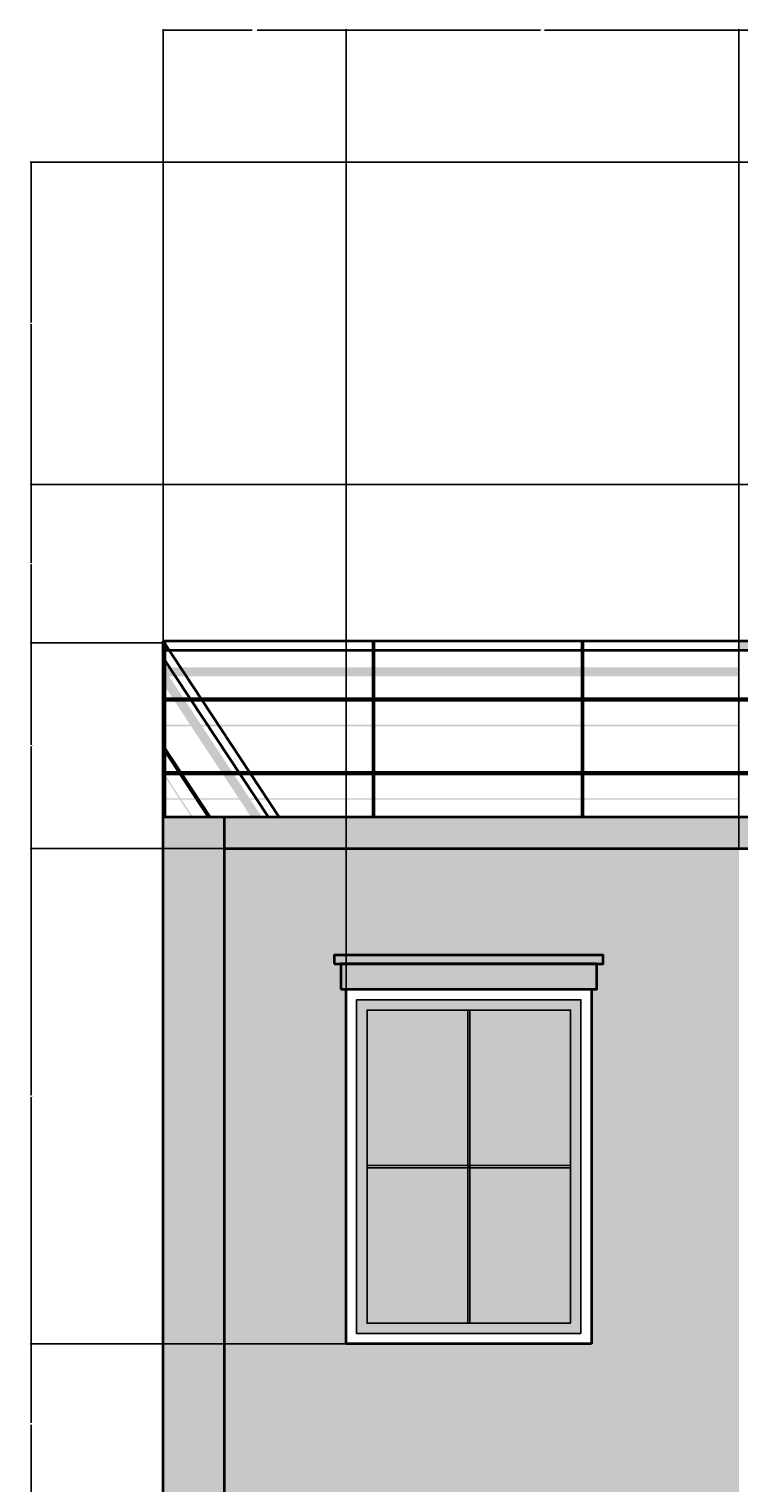
# Model space of a CAD drawing. Units: feet. Extents: x 2415 to 6174, y 866 to 1295.
# Tile 2 of 9: x 3227 to 3364, y 1016 to 1295. Entities that reach past the tile are written whole.
import ezdxf

# ---------------------------------------------------------------- set-up
doc = ezdxf.new("R2010")
doc.units = ezdxf.units.FT
for name, color, linetype, lineweight in [('A-ANNO-DIMS', 2, 'Continuous', 18), ('A-ELEV', 7, 'Continuous', 35), ('A-ELEV-PATT', 8, 'Continuous', 13), ('A-GLAZ', 4, 'Continuous', 25)]:
    doc.layers.add(name, color=color, linetype=linetype, lineweight=lineweight)
doc.styles.get("Standard").update_dxf_attribs({"font": 'arial.ttf'})
doc.dimstyles.get("Standard").update_dxf_attribs({"dimtxt": 0.18, "dimasz": 0.18, "dimexe": 0.18, "dimexo": 0.0625, "dimgap": 0.09, "dimtad": 0, "dimtih": 1, "dimtoh": 1, "dimdec": 1, "dimzin": 0, "dimdsep": 46, "dimlunit": 3, "dimtxsty": 'Standard', "dimcen": 0.09, "dimadec": 0, "dimazin": 0, "dimtfac": 1, "dimtdec": 1, "dimtofl": 0, "dimtmove": 0, "dimatfit": 3, "dimfxl": 1, "dimtolj": 1, "dimtzin": 0, "dimarcsym": 0})

# ---------------------------------------------------------------- blocks, each defined once
blk = doc.blocks.new('WIN-SMALL')
for points in [[(3333.49, 1044.32), (3290.35, 1044.32), (3290.35, 1108.53), (3333.49, 1108.53)], [(3331.49, 1046.32), (3292.35, 1046.32), (3292.35, 1106.53), (3331.49, 1106.53)], [(3311.72, 1106.53), (3312.12, 1106.53), (3312.12, 1046.32), (3311.72, 1046.32)]]:
    blk.add_lwpolyline(points, close=True)
for points in [[(3292.35, 1076.62), (3331.49, 1076.62)], [(3331.49, 1076.22), (3292.35, 1076.22)]]:
    blk.add_lwpolyline(points)
blk = doc.blocks.new('*D61')
at = {"layer": 'A-ANNO-DIMS', "color": 0, "lineweight": -2, "transparency": 16777216}
for p, q in [((3253.13, 1177.2), (3253.13, 1295.18)), ((3253.31, 1295), (3270.27, 1295)), ((3288.17, 1295), (3271.2, 1295)), ((3288.35, 1042.38), (3288.35, 1295.18))]:
    blk.add_line(p, q, dxfattribs=at)
at = {"layer": 'A-ANNO-DIMS', "color": 0, "transparency": 16777216}
for points in [[(3253.31, 1295.03), (3253.31, 1294.97), (3253.13, 1295)], [(3288.17, 1295.03), (3288.17, 1294.97), (3288.35, 1295)]]:
    blk.add_solid(points, dxfattribs=at)
at = {"layer": 'Defpoints', "color": 0, "transparency": 16777216}
for p in [(3288.35, 1295), (3253.13, 1177.14), (3288.35, 1042.32)]:
    blk.add_point(p, dxfattribs=at)
at = {"layer": 'A-ANNO-DIMS', "color": 0, "transparency": 16777216, "insert": (3270.74, 1295), "char_height": 0.18, "attachment_point": 5}
blk.add_mtext('\\A1;35.216', dxfattribs=at)
blk = doc.blocks.new('*D62')
at = {"layer": 'A-ANNO-DIMS', "color": 0, "lineweight": -2, "transparency": 16777216}
for p, q in [((3288.35, 1042.38), (3288.35, 1295.18)), ((3288.53, 1295), (3325.71, 1295)), ((3363.69, 1295), (3326.5, 1295)), ((3363.87, 1137.66), (3363.87, 1295.18))]:
    blk.add_line(p, q, dxfattribs=at)
at = {"layer": 'A-ANNO-DIMS', "color": 0, "transparency": 16777216}
for points in [[(3288.53, 1295.03), (3288.53, 1294.97), (3288.35, 1295)], [(3363.69, 1295.03), (3363.69, 1294.97), (3363.87, 1295)]]:
    blk.add_solid(points, dxfattribs=at)
at = {"layer": 'Defpoints', "color": 0, "transparency": 16777216}
for p in [(3363.87, 1295), (3363.87, 1137.6), (3288.35, 1042.32)]:
    blk.add_point(p, dxfattribs=at)
at = {"layer": 'A-ANNO-DIMS', "color": 0, "transparency": 16777216, "insert": (3326.11, 1295), "char_height": 0.18, "attachment_point": 5}
blk.add_mtext('\\A1;75.52', dxfattribs=at)
blk = doc.blocks.new('*D63')
at = {"layer": 'A-ANNO-DIMS', "color": 0, "lineweight": -2, "transparency": 16777216}
for p, q in [((3363.87, 1137.66), (3363.87, 1295.18)), ((3364.05, 1295), (3414.78, 1295)), ((3466.42, 1295), (3415.69, 1295)), ((3466.6, 1137.66), (3466.6, 1295.18))]:
    blk.add_line(p, q, dxfattribs=at)
at = {"layer": 'A-ANNO-DIMS', "color": 0, "transparency": 16777216}
for points in [[(3364.05, 1295.03), (3364.05, 1294.97), (3363.87, 1295)], [(3466.42, 1295.03), (3466.42, 1294.97), (3466.6, 1295)]]:
    blk.add_solid(points, dxfattribs=at)
at = {"layer": 'Defpoints', "color": 0, "transparency": 16777216}
for p in [(3466.6, 1295), (3363.87, 1137.6), (3466.6, 1137.6)]:
    blk.add_point(p, dxfattribs=at)
at = {"layer": 'A-ANNO-DIMS', "color": 0, "transparency": 16777216, "insert": (3415.23, 1295), "char_height": 0.18, "attachment_point": 5}
blk.add_mtext('\\A1;102.73', dxfattribs=at)
blk = doc.blocks.new('*D74')
at = {"layer": 'A-ANNO-DIMS', "color": 0, "lineweight": -2, "transparency": 16777216}
for p, q in [((3288.28, 1042.32), (3227.55, 1042.32)), ((3227.73, 1042.14), (3227.73, 1027.14)), ((3227.73, 1011.78), (3227.73, 1026.78)), ((3264.85, 1011.6), (3227.55, 1011.6))]:
    blk.add_line(p, q, dxfattribs=at)
at = {"layer": 'A-ANNO-DIMS', "color": 0, "transparency": 16777216}
for points in [[(3227.7, 1042.14), (3227.76, 1042.14), (3227.73, 1042.32)], [(3227.7, 1011.78), (3227.76, 1011.78), (3227.73, 1011.6)]]:
    blk.add_solid(points, dxfattribs=at)
at = {"layer": 'Defpoints', "color": 0, "transparency": 16777216}
for p in [(3227.73, 1042.32), (3288.35, 1042.32), (3264.92, 1011.6)]:
    blk.add_point(p, dxfattribs=at)
at = {"layer": 'A-ANNO-DIMS', "color": 0, "transparency": 16777216, "insert": (3227.73, 1026.96), "char_height": 0.18, "attachment_point": 5}
blk.add_mtext('\\A1;30.72', dxfattribs=at)
blk = doc.blocks.new('*D75')
at = {"layer": 'A-ANNO-DIMS', "color": 0, "lineweight": -2, "transparency": 16777216}
for p, q in [((3363.8, 1137.6), (3227.55, 1137.6)), ((3227.73, 1137.42), (3227.73, 1090.14)), ((3227.73, 1042.5), (3227.73, 1089.78)), ((3288.28, 1042.32), (3227.55, 1042.32))]:
    blk.add_line(p, q, dxfattribs=at)
at = {"layer": 'A-ANNO-DIMS', "color": 0, "transparency": 16777216}
for points in [[(3227.7, 1137.42), (3227.76, 1137.42), (3227.73, 1137.6)], [(3227.7, 1042.5), (3227.76, 1042.5), (3227.73, 1042.32)]]:
    blk.add_solid(points, dxfattribs=at)
at = {"layer": 'Defpoints', "color": 0, "transparency": 16777216}
for p in [(3227.73, 1137.6), (3363.87, 1137.6), (3288.35, 1042.32)]:
    blk.add_point(p, dxfattribs=at)
at = {"layer": 'A-ANNO-DIMS', "color": 0, "transparency": 16777216, "insert": (3227.73, 1089.96), "char_height": 0.18, "attachment_point": 5}
blk.add_mtext('\\A1;95.28', dxfattribs=at)
blk = doc.blocks.new('*D76')
at = {"layer": 'A-ANNO-DIMS', "color": 0, "lineweight": -2, "transparency": 16777216}
for p, q in [((3253.07, 1177.14), (3227.55, 1177.14)), ((3227.73, 1176.96), (3227.73, 1157.55)), ((3227.73, 1137.78), (3227.73, 1157.19)), ((3363.8, 1137.6), (3227.55, 1137.6))]:
    blk.add_line(p, q, dxfattribs=at)
at = {"layer": 'A-ANNO-DIMS', "color": 0, "transparency": 16777216}
for points in [[(3227.7, 1176.96), (3227.76, 1176.96), (3227.73, 1177.14)], [(3227.7, 1137.78), (3227.76, 1137.78), (3227.73, 1137.6)]]:
    blk.add_solid(points, dxfattribs=at)
at = {"layer": 'Defpoints', "color": 0, "transparency": 16777216}
for p in [(3227.73, 1177.14), (3253.13, 1177.14), (3363.87, 1137.6)]:
    blk.add_point(p, dxfattribs=at)
at = {"layer": 'A-ANNO-DIMS', "color": 0, "transparency": 16777216, "insert": (3227.73, 1157.37), "char_height": 0.18, "attachment_point": 5}
blk.add_mtext('\\A1;39.54', dxfattribs=at)
blk = doc.blocks.new('*D77')
at = {"layer": 'A-ANNO-DIMS', "color": 0, "lineweight": -2, "transparency": 16777216}
for p, q in [((3506.73, 1207.6), (3227.55, 1207.6)), ((3227.73, 1207.42), (3227.73, 1192.55)), ((3227.73, 1177.32), (3227.73, 1192.19)), ((3253.07, 1177.14), (3227.55, 1177.14))]:
    blk.add_line(p, q, dxfattribs=at)
at = {"layer": 'A-ANNO-DIMS', "color": 0, "transparency": 16777216}
for points in [[(3227.7, 1207.42), (3227.76, 1207.42), (3227.73, 1207.6)], [(3227.7, 1177.32), (3227.76, 1177.32), (3227.73, 1177.14)]]:
    blk.add_solid(points, dxfattribs=at)
at = {"layer": 'Defpoints', "color": 0, "transparency": 16777216}
for p in [(3227.73, 1207.6), (3506.79, 1207.6), (3253.13, 1177.14)]:
    blk.add_point(p, dxfattribs=at)
at = {"layer": 'A-ANNO-DIMS', "color": 0, "transparency": 16777216, "insert": (3227.73, 1192.37), "char_height": 0.18, "attachment_point": 5}
blk.add_mtext('\\A1;30.457', dxfattribs=at)
blk = doc.blocks.new('*D78')
at = {"layer": 'A-ANNO-DIMS', "color": 0, "lineweight": -2, "transparency": 16777216}
for p, q in [((3571.87, 1269.6), (3227.55, 1269.6)), ((3227.73, 1269.42), (3227.73, 1238.78)), ((3227.73, 1207.78), (3227.73, 1238.42)), ((3506.73, 1207.6), (3227.55, 1207.6))]:
    blk.add_line(p, q, dxfattribs=at)
at = {"layer": 'A-ANNO-DIMS', "color": 0, "transparency": 16777216}
for points in [[(3227.7, 1269.42), (3227.76, 1269.42), (3227.73, 1269.6)], [(3227.7, 1207.78), (3227.76, 1207.78), (3227.73, 1207.6)]]:
    blk.add_solid(points, dxfattribs=at)
at = {"layer": 'Defpoints', "color": 0, "transparency": 16777216}
for p in [(3227.73, 1269.6), (3571.93, 1269.6), (3506.79, 1207.6)]:
    blk.add_point(p, dxfattribs=at)
at = {"layer": 'A-ANNO-DIMS', "color": 0, "transparency": 16777216, "insert": (3227.73, 1238.6), "char_height": 0.18, "attachment_point": 5}
blk.add_mtext('\\A1;62', dxfattribs=at)

msp = doc.modelspace()

# ---------------------------------------------------------------- hatches: boundary and pattern name
at = {"layer": 'A-ELEV-PATT'}
h = msp.add_hatch(color=256, dxfattribs=at)
h.set_gradient(color1=(255, 255, 255), tint=1)
h.paths.add_polyline_path([(3264.916, 1143.5993), (3253.129, 1143.5993), (3253.129, 891.5993), (3264.916, 891.5993)])
h.paths.add_polyline_path([(3470.0448, 1143.5993), (3264.916, 1143.5993), (3264.916, 1137.5992), (3466.5999, 1137.5992)])
h.paths.add_polyline_path([(3363.8667, 1137.5992), (3264.916, 1137.5992), (3264.916, 1011.5992), (3363.8667, 1011.5992)])
h.paths.add_polyline_path([(3286.0429, 1117.0591), (3337.7904, 1117.0591), (3337.7904, 1115.4381), (3336.5314, 1115.4381), (3336.5314, 1110.528), (3335.4882, 1110.528), (3335.4882, 1042.3194), (3288.3452, 1042.3194), (3288.3452, 1110.528), (3287.3019, 1110.528), (3287.3019, 1115.4381), (3286.0429, 1115.4381)], flags=16)
h.paths.add_polyline_path([(3290.3452, 1108.528), (3333.4882, 1108.528), (3333.4882, 1044.3194), (3290.3452, 1044.3194)], flags=0)
h.paths.add_polyline_path([(3292.3452, 1106.528), (3331.4882, 1106.528), (3331.4882, 1046.3194), (3292.3452, 1046.3194)], flags=0)
h.paths.add_polyline_path([(3311.7156, 1106.528), (3312.1178, 1106.528), (3312.1178, 1046.3194), (3311.7156, 1046.3194)], flags=0)
h.paths.add_polyline_path([(3682.0722, 1263.5993), (3578.5579, 1263.5993), (3578.5579, 1137.5992), (3578.5579, 961.3655), (3682.0722, 961.3655)])
h.paths.add_polyline_path([(3660.8129, 1239.0671), (3660.8129, 996.6447), (3602.2151, 996.6447), (3602.2151, 1239.0671)], flags=16)
h.paths.add_polyline_path([(3632.2447, 1239.0671), (3632.2447, 996.6447), (3630.7833, 996.6447), (3630.7833, 1029.3019), (3602.2151, 1029.3019), (3602.2151, 1030.7632), (3630.7833, 1030.7632), (3630.7833, 1071.2549), (3602.2151, 1071.2549), (3602.2151, 1072.7163), (3630.7833, 1072.7163), (3630.7833, 1113.2079), (3602.2151, 1113.2079), (3602.2151, 1114.6693), (3630.7833, 1114.6693), (3630.7833, 1155.161), (3602.2151, 1155.161), (3602.2151, 1156.6224), (3630.7833, 1156.6224), (3630.7833, 1197.114), (3602.2151, 1197.114), (3602.2151, 1198.5754), (3630.7833, 1198.5754), (3630.7833, 1239.0671)], flags=0)
h.paths.add_polyline_path([(3733.129, 951.5993), (3634.5374, 951.5993), (3634.5374, 891.5993), (3733.129, 891.5993)])
h.paths.add_polyline_path([(3627.8799, 951.5993), (3621.0953, 951.5993), (3621.0953, 891.5993), (3627.8799, 891.5993)])
h.paths.add_polyline_path([(3614.4378, 951.5993), (3607.6532, 951.5993), (3607.6532, 891.5993), (3614.4378, 891.5993)])
h.paths.add_polyline_path([(3565.9347, 951.5993), (3441.3079, 951.5993), (3441.3079, 891.5993), (3565.9347, 891.5993)], flags=17)
h.paths.add_polyline_path([(3571.9347, 957.5993), (3435.3079, 957.5993), (3435.3079, 891.5993), (3441.3079, 891.5993), (3441.3079, 951.5993), (3565.9347, 951.5993), (3565.9347, 891.5993), (3571.9347, 891.5993)])
h.paths.add_polyline_path([(3435.3079, 1011.5992), (3423.5209, 1011.5992), (3423.5209, 891.5993), (3435.3079, 891.5993), (3435.3079, 957.5993)])
h.paths.add_polyline_path([(3690.0912, 1269.5992), (3571.9347, 1269.5992), (3571.9347, 1263.5993), (3690.0912, 1263.5993)])
h.paths.add_polyline_path([(3571.9347, 1269.5992), (3538.5122, 1257.6449), (3538.5122, 1251.6449), (3571.9347, 1263.5993)])
h = msp.add_hatch(color=256, dxfattribs=at)
h.set_gradient(color2=(0, 0, 0))
h.paths.add_polyline_path([(3489.4854, 1177.4585), (3454.5146, 1177.4585), (3454.5146, 1175.7117), (3488.4825, 1175.7117)])
h.paths.add_polyline_path([(3454.5146, 1177.4585), (3454.2507, 1177.4585), (3454.2507, 1175.7117), (3454.5146, 1175.7117)])
h.paths.add_polyline_path([(3454.5146, 1175.7117), (3454.2507, 1175.7117), (3454.2507, 1166.3873), (3454.5146, 1166.3873)])
h.paths.add_polyline_path([(3454.5146, 1166.3873), (3454.2507, 1166.3873), (3454.2507, 1166.1234), (3454.5146, 1166.1234)])
h.paths.add_polyline_path([(3483.1288, 1166.3873), (3454.5146, 1166.3873), (3454.5146, 1166.1234), (3482.9773, 1166.1234)])
h.paths.add_polyline_path([(3454.2507, 1166.3873), (3414.3148, 1166.3873), (3414.3148, 1166.1234), (3454.2507, 1166.1234)])
h.paths.add_polyline_path([(3454.5146, 1166.1234), (3454.2507, 1166.1234), (3454.2507, 1152.2269), (3454.5146, 1152.2269)])
h.paths.add_polyline_path([(3454.5146, 1152.2269), (3454.2507, 1152.2269), (3454.2507, 1151.963), (3454.5146, 1151.963)])
h.paths.add_polyline_path([(3474.9985, 1152.2269), (3454.5146, 1152.2269), (3454.5146, 1151.963), (3474.8469, 1151.963)])
h.paths.add_polyline_path([(3454.2507, 1152.2269), (3414.3148, 1152.2269), (3414.3148, 1151.963), (3454.2507, 1151.963)])
h.paths.add_polyline_path([(3454.5146, 1151.963), (3454.2507, 1151.963), (3454.2507, 1143.5993), (3454.5146, 1143.5993)])
h.paths.add_polyline_path([(3414.3148, 1175.7117), (3414.0509, 1175.7117), (3414.0509, 1166.3873), (3414.3148, 1166.3873)])
h.paths.add_polyline_path([(3414.3148, 1166.1234), (3414.0509, 1166.1234), (3414.0509, 1152.2269), (3414.3148, 1152.2269)])
h.paths.add_polyline_path([(3414.3148, 1152.2269), (3414.0509, 1152.2269), (3414.0509, 1151.963), (3414.3148, 1151.963)])
h.paths.add_polyline_path([(3414.3148, 1151.963), (3414.0509, 1151.963), (3414.0509, 1143.5993), (3414.3148, 1143.5993)])
h.paths.add_polyline_path([(3414.0509, 1152.2269), (3374.115, 1152.2269), (3374.115, 1151.963), (3414.0509, 1151.963)])
h.paths.add_polyline_path([(3374.115, 1166.1234), (3373.851, 1166.1234), (3373.851, 1152.2269), (3374.115, 1152.2269)])
h.paths.add_polyline_path([(3374.115, 1151.963), (3373.851, 1151.963), (3373.851, 1143.5993), (3374.115, 1143.5993)])
h.paths.add_polyline_path([(3363.6028, 1172.4585), (3333.9151, 1172.4585), (3333.9151, 1170.7117), (3363.6028, 1170.7117)])
h.paths.add_polyline_path([(3293.4514, 1172.4585), (3253.5155, 1172.4585), (3253.5155, 1171.8725), (3254.2811, 1170.7117), (3293.4514, 1170.7117)])
h.paths.add_polyline_path([(3333.6512, 1172.4585), (3293.7153, 1172.4585), (3293.7153, 1170.7117), (3333.6512, 1170.7117)])
h.paths.add_polyline_path([(3293.7153, 1172.4585), (3293.4514, 1172.4585), (3293.4514, 1170.7117), (3293.7153, 1170.7117)])
h.paths.add_polyline_path([(3333.9151, 1172.4585), (3333.6512, 1172.4585), (3333.6512, 1170.7117), (3333.9151, 1170.7117)])
h.paths.add_polyline_path([(3333.9151, 1170.7117), (3333.6512, 1170.7117), (3333.6512, 1161.3873), (3333.9151, 1161.3873)])
h.paths.add_polyline_path([(3333.9151, 1161.3873), (3333.6512, 1161.3873), (3333.6512, 1161.1234), (3333.9151, 1161.1234)])
h.paths.add_polyline_path([(3363.6028, 1161.3873), (3333.9151, 1161.3873), (3333.9151, 1161.1234), (3363.6028, 1161.1234)])
h.paths.add_polyline_path([(3333.6512, 1161.3873), (3293.7153, 1161.3873), (3293.7153, 1161.1234), (3333.6512, 1161.1234)])
h.paths.add_polyline_path([(3333.9151, 1161.1234), (3333.6512, 1161.1234), (3333.6512, 1147.2269), (3333.9151, 1147.2269)])
h.paths.add_polyline_path([(3333.9151, 1147.2269), (3333.6512, 1147.2269), (3333.6512, 1146.963), (3333.9151, 1146.963)])
h.paths.add_polyline_path([(3333.9151, 1146.963), (3333.6512, 1146.963), (3333.6512, 1143.5993), (3333.9151, 1143.5993)])
h.paths.add_polyline_path([(3363.6028, 1147.2269), (3333.9151, 1147.2269), (3333.9151, 1146.963), (3363.6028, 1146.963)])
h.paths.add_polyline_path([(3333.6512, 1147.2269), (3293.7153, 1147.2269), (3293.7153, 1146.963), (3333.6512, 1146.963)])
h.paths.add_polyline_path([(3293.7153, 1170.7117), (3293.4514, 1170.7117), (3293.4514, 1161.3873), (3293.7153, 1161.3873)])
h.paths.add_polyline_path([(3293.7153, 1161.1234), (3293.4514, 1161.1234), (3293.4514, 1147.2269), (3293.7153, 1147.2269)])
h.paths.add_polyline_path([(3293.7153, 1161.3873), (3293.4514, 1161.3873), (3293.4514, 1161.1234), (3293.7153, 1161.1234)])
h.paths.add_polyline_path([(3293.4514, 1161.3873), (3260.4316, 1161.3873), (3260.6056, 1161.1234), (3293.4514, 1161.1234)])
h.paths.add_polyline_path([(3293.7153, 1147.2269), (3293.4514, 1147.2269), (3293.4514, 1146.963), (3293.7153, 1146.963)])
h.paths.add_polyline_path([(3293.7153, 1146.963), (3293.4514, 1146.963), (3293.4514, 1143.5993), (3293.7153, 1143.5993)])
h.paths.add_polyline_path([(3293.4514, 1147.2269), (3269.7719, 1147.2269), (3269.946, 1146.963), (3293.4514, 1146.963)])
h.paths.add_polyline_path([(3254.2811, 1170.7117), (3253.5155, 1170.7117), (3253.5155, 1168.7002), (3258.3391, 1161.3873), (3260.4316, 1161.3873)])
h.paths.add_polyline_path([(3260.4316, 1161.3873), (3258.3391, 1161.3873), (3258.5131, 1161.1234), (3260.6056, 1161.1234)])
h.paths.add_polyline_path([(3260.6056, 1161.1234), (3258.5131, 1161.1234), (3267.6794, 1147.2269), (3269.7719, 1147.2269)])
h.paths.add_polyline_path([(3258.3391, 1161.3873), (3253.5155, 1161.3873), (3253.5155, 1161.1234), (3258.5131, 1161.1234)])
h.paths.add_polyline_path([(3269.7719, 1147.2269), (3267.6794, 1147.2269), (3267.8535, 1146.963), (3269.946, 1146.963)])
h.paths.add_polyline_path([(3269.946, 1146.963), (3267.8535, 1146.963), (3270.0722, 1143.5993), (3272.1647, 1143.5993)])
h.paths.add_polyline_path([(3267.6794, 1147.2269), (3256.5092, 1147.2269), (3256.6833, 1146.963), (3267.8535, 1146.963)])
h.paths.add_polyline_path([(3256.1931, 1147.2269), (3253.5155, 1147.2269), (3253.5155, 1146.963), (3256.3671, 1146.963)])
h.paths.add_polyline_path([(3253.5155, 1151.7656), (3253.5155, 1151.2863), (3256.1931, 1147.2269), (3256.5092, 1147.2269)])
h.paths.add_polyline_path([(3256.5092, 1147.2269), (3256.1931, 1147.2269), (3256.3671, 1146.963), (3256.6833, 1146.963)])
h.paths.add_polyline_path([(3256.6833, 1146.963), (3256.3671, 1146.963), (3258.5859, 1143.5993), (3258.902, 1143.5993)])
h.paths.add_polyline_path([(3253.2515, 1152.1657), (3253.2515, 1151.6864), (3253.5155, 1151.2863), (3253.5155, 1151.7656)])
h.paths.add_polyline_path([(3253.5155, 1168.7002), (3253.2515, 1169.1003), (3253.2515, 1152.1657), (3253.5155, 1151.7656)])
h.paths.add_polyline_path([(3253.5155, 1151.2863), (3253.2515, 1151.6864), (3253.2515, 1147.2269), (3253.5155, 1147.2269)])
h.paths.add_polyline_path([(3253.5155, 1147.2269), (3253.2515, 1147.2269), (3253.2515, 1146.963), (3253.5155, 1146.963)])
h.paths.add_polyline_path([(3253.5155, 1146.963), (3253.2515, 1146.963), (3253.2515, 1143.5993), (3253.5155, 1143.5993)])
h.paths.add_polyline_path([(3253.5155, 1171.8725), (3253.2515, 1172.2726), (3253.2515, 1169.1003), (3253.5155, 1168.7002)])
h.paths.add_polyline_path([(3253.5155, 1172.4585), (3253.2515, 1172.4585), (3253.2515, 1172.2726), (3253.5155, 1171.8725)])
h.paths.add_polyline_path([(3253.5155, 1171.8725), (3253.5155, 1170.7117), (3254.2811, 1170.7117)], flags=17)
h.paths.add_polyline_path([(3692.5426, 1181.1411), (3682.0722, 1181.1411), (3682.0722, 1179.3943), (3692.5426, 1179.3943)])
h.paths.add_polyline_path([(3732.7425, 1180.5551), (3732.7425, 1181.1411), (3692.8065, 1181.1411), (3692.8065, 1179.3943), (3731.9768, 1179.3943)])
h.paths.add_polyline_path([(3692.8065, 1181.1411), (3692.5426, 1181.1411), (3692.5426, 1179.3943), (3692.8065, 1179.3943)])
h.paths.add_polyline_path([(3692.8065, 1179.3943), (3692.5426, 1179.3943), (3692.5426, 1170.0699), (3692.8065, 1170.0699)])
h.paths.add_polyline_path([(3725.8264, 1170.0699), (3692.8065, 1170.0699), (3692.8065, 1169.806), (3725.6523, 1169.806)])
h.paths.add_polyline_path([(3692.5426, 1170.0699), (3682.0722, 1170.0699), (3682.0722, 1169.806), (3692.5426, 1169.806)])
h.paths.add_polyline_path([(3692.8065, 1170.0699), (3692.5426, 1170.0699), (3692.5426, 1169.806), (3692.8065, 1169.806)])
h.paths.add_polyline_path([(3692.8065, 1169.806), (3692.5426, 1169.806), (3692.5426, 1156.9315), (3692.8065, 1156.9315)])
h.paths.add_polyline_path([(3733.0064, 1180.9552), (3733.0064, 1181.1411), (3732.7425, 1181.1411), (3732.7425, 1180.5551)])
h.paths.add_polyline_path([(3733.0064, 1180.9058), (3732.9836, 1180.9208), (3732.7425, 1180.5551), (3732.7425, 1179.3943), (3733.0064, 1179.3943)])
h.paths.add_polyline_path([(3732.7425, 1180.5551), (3731.9768, 1179.3943), (3732.7425, 1179.3943)], flags=17)
h.paths.add_polyline_path([(3732.7425, 1179.3943), (3731.9768, 1179.3943), (3725.8264, 1170.0699), (3727.9189, 1170.0699), (3732.7425, 1177.3828)])
h.paths.add_polyline_path([(3733.0064, 1179.3943), (3732.7425, 1179.3943), (3732.7425, 1177.3828), (3733.0064, 1177.7829)])
h.paths.add_polyline_path([(3733.0064, 1170.0699), (3732.7425, 1170.0699), (3732.7425, 1169.806), (3733.0064, 1169.806)])
h.paths.add_polyline_path([(3733.0064, 1177.7829), (3732.7425, 1177.3828), (3732.7425, 1170.0699), (3733.0064, 1170.0699)])
h.paths.add_polyline_path([(3732.7425, 1170.0699), (3727.9189, 1170.0699), (3727.7448, 1169.806), (3732.7425, 1169.806)])
h.paths.add_polyline_path([(3727.9189, 1170.0699), (3725.8264, 1170.0699), (3725.6523, 1169.806), (3727.7448, 1169.806)])
h.paths.add_polyline_path([(3727.7448, 1169.806), (3725.6523, 1169.806), (3717.1602, 1156.9315), (3719.2527, 1156.9315)])
h.paths.add_polyline_path([(3733.0064, 1160.369), (3733.0064, 1160.8483), (3732.7425, 1160.4482), (3732.7425, 1159.9689)])
h.paths.add_polyline_path([(3733.0064, 1169.806), (3732.7425, 1169.806), (3732.7425, 1160.4482), (3733.0064, 1160.8483)])
h.paths.add_polyline_path([(3733.0064, 1160.369), (3732.7425, 1159.9689), (3732.7425, 1156.9315), (3733.0064, 1156.9315)])
h = msp.add_hatch(color=256, dxfattribs=at)
h.set_gradient(color2=(0, 0, 0))
h.paths.add_polyline_path([(3373.851, 1177.4585), (3363.8667, 1177.4585), (3363.8667, 1175.7117), (3373.851, 1175.7117)])
h.paths.add_polyline_path([(3374.115, 1177.4585), (3373.851, 1177.4585), (3373.851, 1175.7117), (3374.115, 1175.7117)])
h.paths.add_polyline_path([(3414.0509, 1177.4585), (3374.115, 1177.4585), (3374.115, 1175.7117), (3414.0509, 1175.7117)])
h.paths.add_polyline_path([(3414.3148, 1177.4585), (3414.0509, 1177.4585), (3414.0509, 1175.7117), (3414.3148, 1175.7117)])
h.paths.add_polyline_path([(3363.8667, 1177.4585), (3363.6028, 1177.4585), (3363.6028, 1172.4585), (3363.8667, 1172.4585)])
h.paths.add_polyline_path([(3363.8667, 1172.4585), (3363.6028, 1172.4585), (3363.6028, 1170.7117), (3363.8667, 1170.7117)])
h.paths.add_polyline_path([(3363.8667, 1170.7117), (3363.6028, 1170.7117), (3363.6028, 1161.3873), (3363.8667, 1161.3873)])
h.paths.add_polyline_path([(3363.8667, 1161.3873), (3363.6028, 1161.3873), (3363.6028, 1161.1234), (3363.8667, 1161.1234)])
h.paths.add_polyline_path([(3363.8667, 1161.1234), (3363.6028, 1161.1234), (3363.6028, 1147.2269), (3363.8667, 1147.2269)])
h.paths.add_polyline_path([(3363.8667, 1147.2269), (3363.6028, 1147.2269), (3363.6028, 1146.963), (3363.8667, 1146.963)])
h.paths.add_polyline_path([(3363.8667, 1146.963), (3363.6028, 1146.963), (3363.6028, 1143.5993), (3363.8667, 1143.5993)])
h.paths.add_polyline_path([(3373.851, 1152.2269), (3363.8667, 1152.2269), (3363.8667, 1151.963), (3373.851, 1151.963)])
h.paths.add_polyline_path([(3374.115, 1152.2269), (3373.851, 1152.2269), (3373.851, 1151.963), (3374.115, 1151.963)])
h.paths.add_polyline_path([(3374.115, 1175.7117), (3373.851, 1175.7117), (3373.851, 1166.3873), (3374.115, 1166.3873)])
h.paths.add_polyline_path([(3373.851, 1166.3873), (3363.8667, 1166.3873), (3363.8667, 1166.1234), (3373.851, 1166.1234)])
h.paths.add_polyline_path([(3374.115, 1166.3873), (3373.851, 1166.3873), (3373.851, 1166.1234), (3374.115, 1166.1234)])
h.paths.add_polyline_path([(3414.0509, 1166.3873), (3374.115, 1166.3873), (3374.115, 1166.1234), (3414.0509, 1166.1234)])
h = msp.add_hatch(color=256, dxfattribs=at)
h.set_gradient(color1=(99, 100, 102), color2=(99, 100, 102))
h.paths.add_polyline_path([(3336.5314, 1115.4381), (3287.3019, 1115.4381), (3287.3019, 1110.528), (3336.5314, 1110.528)])
h.paths.add_polyline_path([(3337.7904, 1117.0591), (3286.0429, 1117.0591), (3286.0429, 1115.4381), (3337.7904, 1115.4381)])
h = msp.add_hatch(color=256, dxfattribs=at)
h.set_gradient(color1=(199, 200, 202), color2=(173, 221, 247))
h.paths.add_polyline_path([(3331.4882, 1106.528), (3312.1178, 1106.528), (3312.1178, 1076.6248), (3331.4882, 1076.6248)])
h.paths.add_polyline_path([(3331.4882, 1076.2226), (3312.1178, 1076.2226), (3312.1178, 1046.3194), (3331.4882, 1046.3194)])
h.paths.add_polyline_path([(3311.7156, 1076.2226), (3292.3452, 1076.2226), (3292.3452, 1046.3194), (3311.7156, 1046.3194)])
h.paths.add_polyline_path([(3311.7156, 1106.528), (3292.3452, 1106.528), (3292.3452, 1076.6248), (3311.7156, 1076.6248)])

# ---------------------------------------------------------------- linework, layer by layer
at = {"layer": 'A-ELEV'}
for p, q in [((3253.129, 1143.5993), (3253.129, 1177.4585)), ((3253.129, 1177.4585), (3275.4627, 1143.5993)), ((3253.129, 891.5993), (3253.129, 1143.5993)), ((3264.916, 1143.5993), (3253.129, 1143.5993)), ((3470.0448, 1143.5993), (3264.916, 1143.5993)), ((3264.916, 1137.5992), (3578.5579, 1137.5992))]:
    msp.add_line(p, q, dxfattribs=at)
for points in [[(3489.4854, 1177.4585), (3253.129, 1177.4585)], [(3253.129, 1177.1423), (3253.2743, 1177.2382)], [(3253.2515, 1177.4585), (3253.2515, 1143.5993)], [(3253.5155, 1143.5993), (3253.5155, 1177.4585)], [(3293.4514, 1177.4585), (3293.4514, 1143.5993)], [(3293.7153, 1143.5993), (3293.7153, 1177.4585)], [(3333.6512, 1177.4585), (3333.6512, 1143.5993)], [(3333.9151, 1143.5993), (3333.9151, 1177.4585)], [(3253.129, 1175.7117), (3488.4825, 1175.7117)], [(3253.129, 1174.2861), (3273.3702, 1143.5993)], [(3483.1288, 1166.3873), (3253.129, 1166.3873)], [(3253.129, 1166.1234), (3482.9773, 1166.1234)], [(3262.2001, 1143.5993), (3253.129, 1157.3516)], [(3253.129, 1156.8722), (3261.8839, 1143.5993)], [(3474.9985, 1152.2269), (3253.129, 1152.2269)], [(3253.129, 1151.963), (3474.8469, 1151.963)], [(3253.129, 891.5993), (3264.916, 891.5993), (3264.916, 1143.5993)], [(3275.2635, 1143.9012), (3274.8057, 1143.5993)], [(3275.285, 1143.5993), (3275.4088, 1143.6809)]]:
    msp.add_lwpolyline(points, dxfattribs=at)
for points in [[(3286.0429, 1115.4381), (3337.7904, 1115.4381), (3337.7904, 1117.0591), (3286.0429, 1117.0591)], [(3287.3019, 1110.528), (3336.5314, 1110.528), (3336.5314, 1115.4381), (3287.3019, 1115.4381)], [(3335.4882, 1042.3194), (3288.3452, 1042.3194), (3288.3452, 1110.528), (3335.4882, 1110.528)]]:
    msp.add_lwpolyline(points, close=True, dxfattribs=at)

# ---------------------------------------------------------------- block references
at = {"layer": 'A-GLAZ'}
msp.add_blockref('WIN-SMALL', (0, 0), dxfattribs=at)

# ---------------------------------------------------------------- dimensions: what is measured, and where the dimension line sits
at = {"layer": 'A-ANNO-DIMS'}
for base, p1, p2, override, picture, middle in [((3288.3452, 1294.9993), (3253.129, 1177.1423), (3288.3452, 1042.3194), {"dimdec": 3, "dimlfac": 1, "dimrnd": 0, "dimzin": 0, "dimdsep": 46, "dimlunit": 2}, '*D61', (3270.7371, 1294.9993)), ((3363.8667, 1294.9993), (3288.3452, 1042.3194), (3363.8667, 1137.5992), {"dimdec": 2, "dimlfac": 1, "dimrnd": 0, "dimzin": 0, "dimdsep": 46, "dimlunit": 2}, '*D62', (3326.106, 1294.9993)), ((3466.5999, 1294.9993), (3363.8667, 1137.5992), (3466.5999, 1137.5992), {"dimdec": 2, "dimlfac": 1, "dimrnd": 0, "dimzin": 0, "dimdsep": 46, "dimlunit": 2}, '*D63', (3415.2333, 1294.9993))]:
    dim = msp.add_linear_dim(base=base, p1=p1, p2=p2, dimstyle='Standard', override=override, dxfattribs=at)
    dim.commit()
    dim.dimension.update_dxf_attribs({"geometry": picture, "text_midpoint": middle})
for base, p1, p2, override, picture, middle in [((3227.729, 1269.5992), (3506.791, 1207.5992), (3571.9347, 1269.5992), {"dimdec": 0, "dimlfac": 1, "dimrnd": 0, "dimzin": 0, "dimdsep": 46, "dimlunit": 2}, '*D78', (3227.729, 1238.5992)), ((3227.729, 1207.5992), (3253.129, 1177.1423), (3506.791, 1207.5992), {"dimdec": 3, "dimlfac": 1, "dimrnd": 0, "dimzin": 0, "dimdsep": 46, "dimlunit": 2}, '*D77', (3227.729, 1192.3708)), ((3227.729, 1177.1423), (3363.8667, 1137.5992), (3253.129, 1177.1423), {"dimdec": 2, "dimlfac": 1, "dimrnd": 0, "dimzin": 0, "dimdsep": 46, "dimlunit": 2}, '*D76', (3227.729, 1157.3708)), ((3227.729, 1137.5992), (3288.3452, 1042.3194), (3363.8667, 1137.5992), {"dimdec": 2, "dimlfac": 1, "dimrnd": 0, "dimzin": 0, "dimdsep": 46, "dimlunit": 2}, '*D75', (3227.729, 1089.9593)), ((3227.729, 1042.3194), (3264.916, 1011.5992), (3288.3452, 1042.3194), {"dimdec": 2, "dimlfac": 1, "dimrnd": 0, "dimzin": 0, "dimdsep": 46, "dimlunit": 2}, '*D74', (3227.729, 1026.9593))]:
    dim = msp.add_linear_dim(base=base, p1=p1, p2=p2, angle=90, dimstyle='Standard', override=override, dxfattribs=at)
    dim.commit()
    dim.dimension.update_dxf_attribs({"geometry": picture, "text_midpoint": middle})

doc.saveas('drawing.dxf')
